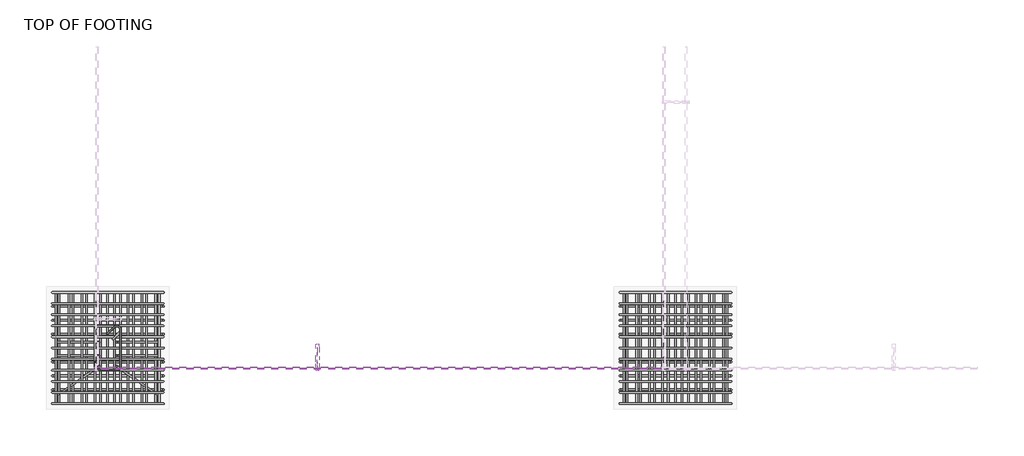
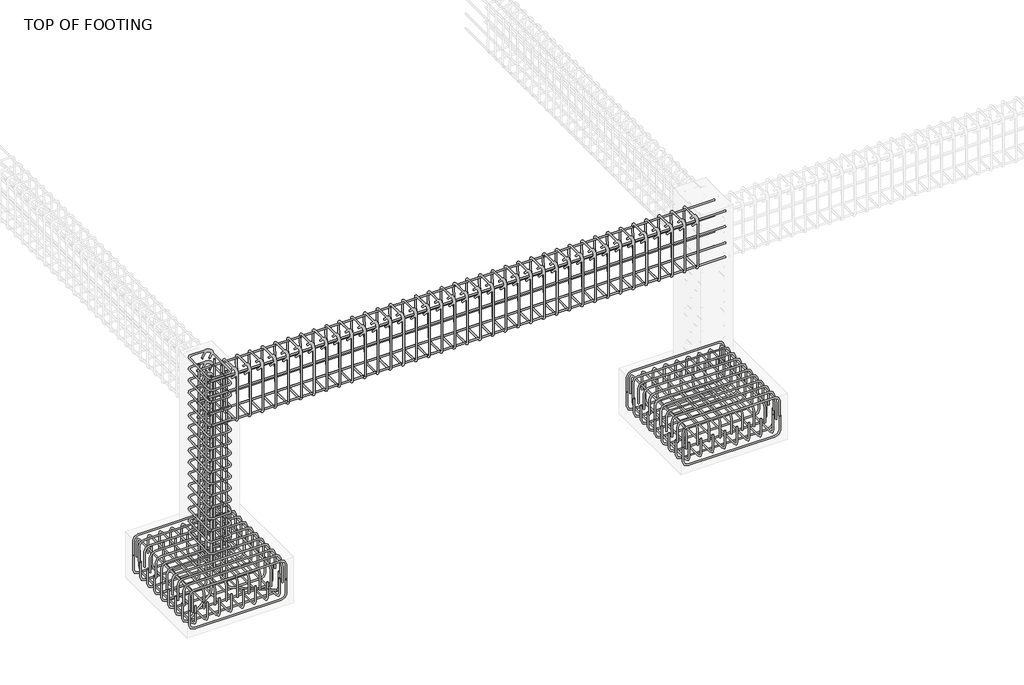
# One storey, part 2 of 13: 18 reinforcing bars.
"""IFC4 building model written with IfcOpenShell, lengths in millimetres."""

from ifc_helpers import new_model, si_unit, point, frame, origin, place, context, project, spatial, polyline, circle_curve, trimmed, segment, composite_curve, source, transform, mapped, element, save
from ifc_brep_helpers import swept_disk

model = new_model("IFC4")

# Units and contexts
model_context = context("Model", 3, world=origin())
ifc_project = project(units=[si_unit("LENGTHUNIT", "METRE", prefix="MILLI")], contexts=[model_context])

# Site, building, storey
site = spatial("IfcSite", under=ifc_project)
building = spatial("IfcBuilding", under=site)
storey = spatial("IfcBuildingStorey", under=building, Name="TOP OF FOOTING", Elevation=-1828.8)

# Reinforcing bars
placement = place(None, origin())
reinforcing_bar_shape = source(origin(), model_context, "Body", "SolidModel", [
    swept_disk(composite_curve([segment(polyline([(-6869.8542006, -3805.7842236, -2046.7304597), (-6869.8542006, -3805.7842236, -2194.0304597)]), True, "CONTINUOUS"), segment(trimmed(circle_curve(frame((-6916.2042006, -3805.7842236, -2194.0304597), z_axis=(0.0, 1.0, 0.0), x_axis=(46.350000000000364, 0.0, 0.0)), 46.35), [point((-6869.8542006, -3805.7842236, -2194.0304597))], [point((-6916.2042006, -3805.7842236, -2240.3804597))], True, "CARTESIAN"), True, "CONTINUOUS"), segment(polyline([(-6916.2042006, -3805.7842236, -2240.3804597), (-7730.8042006, -3805.7842236, -2240.3804597)]), True, "CONTINUOUS"), segment(trimmed(circle_curve(frame((-7730.8042006, -3805.7842236, -2194.0304597), z_axis=(0.0, 1.0, 0.0), x_axis=(0.0, 0.0, -46.34999999999991)), 46.35), [point((-7730.8042006, -3805.7842236, -2240.3804597))], [point((-7777.1542006, -3805.7842236, -2194.0304597))], True, "CARTESIAN"), True, "CONTINUOUS"), segment(polyline([(-7777.1542006, -3805.7842236, -2194.0304597), (-7777.1542006, -3805.7842236, -2046.7304597)]), True, "CONTINUOUS")], self_intersect=False), 6.35),
])
element("IfcReinforcingBar", 1, at=placement, inside=storey, context=model_context, shape_type="MappedRepresentation", body=[
    mapped(reinforcing_bar_shape, transform((0.0, 0.0, 0.0), x_axis=(1.0, 0.0, 0.0), y_axis=(0.0, 1.0, 0.0), z_axis=(0.0, 0.0, 1.0))),
    mapped(reinforcing_bar_shape, transform((0.0, -113.4125, 0.0), x_axis=(1.0, 0.0, 0.0), y_axis=(0.0, 1.0, 0.0), z_axis=(0.0, 0.0, 1.0))),
    mapped(reinforcing_bar_shape, transform((0.0, -226.825, 0.0), x_axis=(1.0, 0.0, 0.0), y_axis=(0.0, 1.0, 0.0), z_axis=(0.0, 0.0, 1.0))),
    mapped(reinforcing_bar_shape, transform((0.0, -340.2375, 0.0), x_axis=(1.0, 0.0, 0.0), y_axis=(0.0, 1.0, 0.0), z_axis=(0.0, 0.0, 1.0))),
    mapped(reinforcing_bar_shape, transform((0.0, -453.65, 0.0), x_axis=(1.0, 0.0, 0.0), y_axis=(0.0, 1.0, 0.0), z_axis=(0.0, 0.0, 1.0))),
    mapped(reinforcing_bar_shape, transform((0.0, -567.0625, 0.0), x_axis=(1.0, 0.0, 0.0), y_axis=(0.0, 1.0, 0.0), z_axis=(0.0, 0.0, 1.0))),
    mapped(reinforcing_bar_shape, transform((0.0, -680.475, 0.0), x_axis=(1.0, 0.0, 0.0), y_axis=(0.0, 1.0, 0.0), z_axis=(0.0, 0.0, 1.0))),
    mapped(reinforcing_bar_shape, transform((0.0, -793.8875, 0.0), x_axis=(1.0, 0.0, 0.0), y_axis=(0.0, 1.0, 0.0), z_axis=(0.0, 0.0, 1.0))),
    mapped(reinforcing_bar_shape, transform((0.0, -907.3, 0.0), x_axis=(1.0, 0.0, 0.0), y_axis=(0.0, 1.0, 0.0), z_axis=(0.0, 0.0, 1.0))),
])
reinforcing_bar_2_shape = source(origin(), model_context, "Body", "SolidModel", [
    swept_disk(composite_curve([segment(polyline([(-7777.3413042, -3805.7842236, -2054.7114114), (-7777.3413042, -3805.7842236, -1907.4114114)]), True, "CONTINUOUS"), segment(trimmed(circle_curve(frame((-7730.9913042, -3805.7842236, -1907.4114114), z_axis=(0.0, 1.0, 0.0), x_axis=(-46.350000000000364, 0.0, 0.0)), 46.35), [point((-7777.3413042, -3805.7842236, -1907.4114114))], [point((-7730.9913042, -3805.7842236, -1861.0614114))], True, "CARTESIAN"), True, "CONTINUOUS"), segment(polyline([(-7730.9913042, -3805.7842236, -1861.0614114), (-6918.3621718, -3805.7842236, -1861.0614114)]), True, "CONTINUOUS"), segment(trimmed(circle_curve(frame((-6918.3621718, -3805.7842236, -1907.4114114), z_axis=(0.0, 1.0, 0.0), x_axis=(0.0, 0.0, 46.34999999999991)), 46.35), [point((-6918.3621718, -3805.7842236, -1861.0614114))], [point((-6872.0121718, -3805.7842236, -1907.4114114))], True, "CARTESIAN"), True, "CONTINUOUS"), segment(polyline([(-6872.0121718, -3805.7842236, -1907.4114114), (-6872.0121718, -3805.7842236, -2054.7114114)]), True, "CONTINUOUS")], self_intersect=False), 6.35),
])
element("IfcReinforcingBar", 2, at=placement, inside=storey, context=model_context, shape_type="MappedRepresentation", body=[
    mapped(reinforcing_bar_2_shape, transform((0.0, 0.0, 0.0), x_axis=(1.0, 0.0, 0.0), y_axis=(0.0, 1.0, 0.0), z_axis=(0.0, 0.0, 1.0))),
    mapped(reinforcing_bar_2_shape, transform((0.0, -90.73, 0.0), x_axis=(1.0, 0.0, 0.0), y_axis=(0.0, 1.0, 0.0), z_axis=(0.0, 0.0, 1.0))),
    mapped(reinforcing_bar_2_shape, transform((0.0, -181.46, 0.0), x_axis=(1.0, 0.0, 0.0), y_axis=(0.0, 1.0, 0.0), z_axis=(0.0, 0.0, 1.0))),
    mapped(reinforcing_bar_2_shape, transform((0.0, -272.19, 0.0), x_axis=(1.0, 0.0, 0.0), y_axis=(0.0, 1.0, 0.0), z_axis=(0.0, 0.0, 1.0))),
    mapped(reinforcing_bar_2_shape, transform((0.0, -362.92, 0.0), x_axis=(1.0, 0.0, 0.0), y_axis=(0.0, 1.0, 0.0), z_axis=(0.0, 0.0, 1.0))),
    mapped(reinforcing_bar_2_shape, transform((0.0, -453.65, 0.0), x_axis=(1.0, 0.0, 0.0), y_axis=(0.0, 1.0, 0.0), z_axis=(0.0, 0.0, 1.0))),
    mapped(reinforcing_bar_2_shape, transform((0.0, -544.38, 0.0), x_axis=(1.0, 0.0, 0.0), y_axis=(0.0, 1.0, 0.0), z_axis=(0.0, 0.0, 1.0))),
    mapped(reinforcing_bar_2_shape, transform((0.0, -635.11, 0.0), x_axis=(1.0, 0.0, 0.0), y_axis=(0.0, 1.0, 0.0), z_axis=(0.0, 0.0, 1.0))),
    mapped(reinforcing_bar_2_shape, transform((0.0, -725.84, 0.0), x_axis=(1.0, 0.0, 0.0), y_axis=(0.0, 1.0, 0.0), z_axis=(0.0, 0.0, 1.0))),
    mapped(reinforcing_bar_2_shape, transform((0.0, -816.57, 0.0), x_axis=(1.0, 0.0, 0.0), y_axis=(0.0, 1.0, 0.0), z_axis=(0.0, 0.0, 1.0))),
    mapped(reinforcing_bar_2_shape, transform((0.0, -907.3, 0.0), x_axis=(1.0, 0.0, 0.0), y_axis=(0.0, 1.0, 0.0), z_axis=(0.0, 0.0, 1.0))),
])
reinforcing_bar_3_shape = source(origin(), model_context, "Body", "SolidModel", [
    swept_disk(composite_curve([segment(polyline([(-7721.4502846, -3805.7842236, -2022.6645135), (-7721.4502846, -3805.7842236, -2169.9645135)]), True, "CONTINUOUS"), segment(trimmed(circle_curve(frame((-7721.4502846, -3852.1342236, -2169.9645135), z_axis=(-1.0, 0.0, 0.0), x_axis=(0.0, 46.34999999999991, 0.0)), 46.35), [point((-7721.4502846, -3805.7842236, -2169.9645135))], [point((-7721.4502846, -3852.1342236, -2216.3145135))], True, "CARTESIAN"), True, "CONTINUOUS"), segment(polyline([(-7721.4502846, -3852.1342236, -2216.3145135), (-7721.4502846, -4666.7342236, -2216.3145135)]), True, "CONTINUOUS"), segment(trimmed(circle_curve(frame((-7721.4502846, -4666.7342236, -2169.9645135), z_axis=(-1.0, 0.0, 0.0), x_axis=(0.0, 0.0, -46.34999999999991)), 46.35), [point((-7721.4502846, -4666.7342236, -2216.3145135))], [point((-7721.4502846, -4713.0842236, -2169.9645135))], True, "CARTESIAN"), True, "CONTINUOUS"), segment(polyline([(-7721.4502846, -4713.0842236, -2169.9645135), (-7721.4502846, -4713.0842236, -2022.6645135)]), True, "CONTINUOUS")], self_intersect=False), 6.35),
])
element("IfcReinforcingBar", 3, at=placement, inside=storey, context=model_context, shape_type="MappedRepresentation", body=[
    mapped(reinforcing_bar_3_shape, transform((0.0, 0.0, 0.0), x_axis=(1.0, 0.0, 0.0), y_axis=(0.0, 1.0, 0.0), z_axis=(0.0, 0.0, 1.0))),
    mapped(reinforcing_bar_3_shape, transform((112.5551949, 0.0, 0.0), x_axis=(1.0, 0.0, 0.0), y_axis=(0.0, 1.0, 0.0), z_axis=(0.0, 0.0, 1.0))),
    mapped(reinforcing_bar_3_shape, transform((225.1103897, 0.0, 0.0), x_axis=(1.0, 0.0, 0.0), y_axis=(0.0, 1.0, 0.0), z_axis=(0.0, 0.0, 1.0))),
    mapped(reinforcing_bar_3_shape, transform((337.6655846, 0.0, 0.0), x_axis=(1.0, 0.0, 0.0), y_axis=(0.0, 1.0, 0.0), z_axis=(0.0, 0.0, 1.0))),
    mapped(reinforcing_bar_3_shape, transform((450.2207794, 0.0, 0.0), x_axis=(1.0, 0.0, 0.0), y_axis=(0.0, 1.0, 0.0), z_axis=(0.0, 0.0, 1.0))),
    mapped(reinforcing_bar_3_shape, transform((562.7759743, 0.0, 0.0), x_axis=(1.0, 0.0, 0.0), y_axis=(0.0, 1.0, 0.0), z_axis=(0.0, 0.0, 1.0))),
    mapped(reinforcing_bar_3_shape, transform((675.3311691, 0.0, 0.0), x_axis=(1.0, 0.0, 0.0), y_axis=(0.0, 1.0, 0.0), z_axis=(0.0, 0.0, 1.0))),
    mapped(reinforcing_bar_3_shape, transform((787.886364, 0.0, 0.0), x_axis=(1.0, 0.0, 0.0), y_axis=(0.0, 1.0, 0.0), z_axis=(0.0, 0.0, 1.0))),
])
reinforcing_bar_4_shape = source(origin(), model_context, "Body", "SolidModel", [
    swept_disk(composite_curve([segment(polyline([(-6905.0104502, -3805.7842236, -2073.3758937), (-6905.0104502, -3805.7842236, -1926.0758937)]), True, "CONTINUOUS"), segment(trimmed(circle_curve(frame((-6905.0104502, -3852.1342236, -1926.0758937), z_axis=(1.0, 0.0, 0.0), x_axis=(0.0, 46.34999999999991, 0.0)), 46.35), [point((-6905.0104502, -3805.7842236, -1926.0758937))], [point((-6905.0104502, -3852.1342236, -1879.7258937))], True, "CARTESIAN"), True, "CONTINUOUS"), segment(polyline([(-6905.0104502, -3852.1342236, -1879.7258937), (-6905.0104502, -4666.7342236, -1879.7258937)]), True, "CONTINUOUS"), segment(trimmed(circle_curve(frame((-6905.0104502, -4666.7342236, -1926.0758937), z_axis=(1.0, 0.0, 0.0), x_axis=(0.0, 0.0, 46.350000000000136)), 46.35), [point((-6905.0104502, -4666.7342236, -1879.7258937))], [point((-6905.0104502, -4713.0842236, -1926.0758937))], True, "CARTESIAN"), True, "CONTINUOUS"), segment(polyline([(-6905.0104502, -4713.0842236, -1926.0758937), (-6905.0104502, -4713.0842236, -2073.3758937)]), True, "CONTINUOUS")], self_intersect=False), 6.35),
])
element("IfcReinforcingBar", 4, at=placement, inside=storey, context=model_context, shape_type="MappedRepresentation", body=[
    mapped(reinforcing_bar_4_shape, transform((0.0, 0.0, 0.0), x_axis=(1.0, 0.0, 0.0), y_axis=(0.0, 1.0, 0.0), z_axis=(0.0, 0.0, 1.0))),
    mapped(reinforcing_bar_4_shape, transform((-105.0563863, 0.0, 0.0), x_axis=(1.0, 0.0, 0.0), y_axis=(0.0, 1.0, 0.0), z_axis=(0.0, 0.0, 1.0))),
    mapped(reinforcing_bar_4_shape, transform((-210.1127725, 0.0, 0.0), x_axis=(1.0, 0.0, 0.0), y_axis=(0.0, 1.0, 0.0), z_axis=(0.0, 0.0, 1.0))),
    mapped(reinforcing_bar_4_shape, transform((-315.1691588, 0.0, 0.0), x_axis=(1.0, 0.0, 0.0), y_axis=(0.0, 1.0, 0.0), z_axis=(0.0, 0.0, 1.0))),
    mapped(reinforcing_bar_4_shape, transform((-420.2255451, 0.0, 0.0), x_axis=(1.0, 0.0, 0.0), y_axis=(0.0, 1.0, 0.0), z_axis=(0.0, 0.0, 1.0))),
    mapped(reinforcing_bar_4_shape, transform((-525.2819314, 0.0, 0.0), x_axis=(1.0, 0.0, 0.0), y_axis=(0.0, 1.0, 0.0), z_axis=(0.0, 0.0, 1.0))),
    mapped(reinforcing_bar_4_shape, transform((-630.3383176, 0.0, 0.0), x_axis=(1.0, 0.0, 0.0), y_axis=(0.0, 1.0, 0.0), z_axis=(0.0, 0.0, 1.0))),
    mapped(reinforcing_bar_4_shape, transform((-735.3947039, 0.0, 0.0), x_axis=(1.0, 0.0, 0.0), y_axis=(0.0, 1.0, 0.0), z_axis=(0.0, 0.0, 1.0))),
    mapped(reinforcing_bar_4_shape, transform((-840.4510902, 0.0, 0.0), x_axis=(1.0, 0.0, 0.0), y_axis=(0.0, 1.0, 0.0), z_axis=(0.0, 0.0, 1.0))),
])
reinforcing_bar_5_shape = source(origin(), model_context, "Body", "SolidModel", [
    swept_disk(composite_curve([segment(polyline([(-2242.1090063, -3805.7842236, -2046.7304597), (-2242.1090063, -3805.7842236, -2194.0304597)]), True, "CONTINUOUS"), segment(trimmed(circle_curve(frame((-2288.4590063, -3805.7842236, -2194.0304597), z_axis=(0.0, 1.0, 0.0), x_axis=(46.34999999999991, 0.0, 0.0)), 46.35), [point((-2242.1090063, -3805.7842236, -2194.0304597))], [point((-2288.4590063, -3805.7842236, -2240.3804597))], True, "CARTESIAN"), True, "CONTINUOUS"), segment(polyline([(-2288.4590063, -3805.7842236, -2240.3804597), (-3103.0590063, -3805.7842236, -2240.3804597)]), True, "CONTINUOUS"), segment(trimmed(circle_curve(frame((-3103.0590063, -3805.7842236, -2194.0304597), z_axis=(0.0, 1.0, 0.0), x_axis=(0.0, 0.0, -46.34999999999991)), 46.35), [point((-3103.0590063, -3805.7842236, -2240.3804597))], [point((-3149.4090063, -3805.7842236, -2194.0304597))], True, "CARTESIAN"), True, "CONTINUOUS"), segment(polyline([(-3149.4090063, -3805.7842236, -2194.0304597), (-3149.4090063, -3805.7842236, -2046.7304597)]), True, "CONTINUOUS")], self_intersect=False), 6.35),
])
element("IfcReinforcingBar", 5, at=placement, inside=storey, context=model_context, shape_type="MappedRepresentation", body=[
    mapped(reinforcing_bar_5_shape, transform((0.0, 0.0, 0.0), x_axis=(1.0, 0.0, 0.0), y_axis=(0.0, 1.0, 0.0), z_axis=(0.0, 0.0, 1.0))),
    mapped(reinforcing_bar_5_shape, transform((0.0, -113.4125, 0.0), x_axis=(1.0, 0.0, 0.0), y_axis=(0.0, 1.0, 0.0), z_axis=(0.0, 0.0, 1.0))),
    mapped(reinforcing_bar_5_shape, transform((0.0, -226.825, 0.0), x_axis=(1.0, 0.0, 0.0), y_axis=(0.0, 1.0, 0.0), z_axis=(0.0, 0.0, 1.0))),
    mapped(reinforcing_bar_5_shape, transform((0.0, -340.2375, 0.0), x_axis=(1.0, 0.0, 0.0), y_axis=(0.0, 1.0, 0.0), z_axis=(0.0, 0.0, 1.0))),
    mapped(reinforcing_bar_5_shape, transform((0.0, -453.65, 0.0), x_axis=(1.0, 0.0, 0.0), y_axis=(0.0, 1.0, 0.0), z_axis=(0.0, 0.0, 1.0))),
    mapped(reinforcing_bar_5_shape, transform((0.0, -567.0625, 0.0), x_axis=(1.0, 0.0, 0.0), y_axis=(0.0, 1.0, 0.0), z_axis=(0.0, 0.0, 1.0))),
    mapped(reinforcing_bar_5_shape, transform((0.0, -680.475, 0.0), x_axis=(1.0, 0.0, 0.0), y_axis=(0.0, 1.0, 0.0), z_axis=(0.0, 0.0, 1.0))),
    mapped(reinforcing_bar_5_shape, transform((0.0, -793.8875, 0.0), x_axis=(1.0, 0.0, 0.0), y_axis=(0.0, 1.0, 0.0), z_axis=(0.0, 0.0, 1.0))),
    mapped(reinforcing_bar_5_shape, transform((0.0, -907.3, 0.0), x_axis=(1.0, 0.0, 0.0), y_axis=(0.0, 1.0, 0.0), z_axis=(0.0, 0.0, 1.0))),
])
reinforcing_bar_6_shape = source(origin(), model_context, "Body", "SolidModel", [
    swept_disk(composite_curve([segment(polyline([(-3149.5961099, -3805.7842236, -2054.7114114), (-3149.5961099, -3805.7842236, -1907.4114114)]), True, "CONTINUOUS"), segment(trimmed(circle_curve(frame((-3103.2461099, -3805.7842236, -1907.4114114), z_axis=(0.0, 1.0, 0.0), x_axis=(-46.34999999999991, 0.0, 0.0)), 46.35), [point((-3149.5961099, -3805.7842236, -1907.4114114))], [point((-3103.2461099, -3805.7842236, -1861.0614114))], True, "CARTESIAN"), True, "CONTINUOUS"), segment(polyline([(-3103.2461099, -3805.7842236, -1861.0614114), (-2290.6169775, -3805.7842236, -1861.0614114)]), True, "CONTINUOUS"), segment(trimmed(circle_curve(frame((-2290.6169775, -3805.7842236, -1907.4114114), z_axis=(0.0, 1.0, 0.0), x_axis=(0.0, 0.0, 46.34999999999991)), 46.35), [point((-2290.6169775, -3805.7842236, -1861.0614114))], [point((-2244.2669775, -3805.7842236, -1907.4114114))], True, "CARTESIAN"), True, "CONTINUOUS"), segment(polyline([(-2244.2669775, -3805.7842236, -1907.4114114), (-2244.2669775, -3805.7842236, -2054.7114114)]), True, "CONTINUOUS")], self_intersect=False), 6.35),
])
element("IfcReinforcingBar", 6, at=placement, inside=storey, context=model_context, shape_type="MappedRepresentation", body=[
    mapped(reinforcing_bar_6_shape, transform((0.0, 0.0, 0.0), x_axis=(1.0, 0.0, 0.0), y_axis=(0.0, 1.0, 0.0), z_axis=(0.0, 0.0, 1.0))),
    mapped(reinforcing_bar_6_shape, transform((0.0, -90.73, 0.0), x_axis=(1.0, 0.0, 0.0), y_axis=(0.0, 1.0, 0.0), z_axis=(0.0, 0.0, 1.0))),
    mapped(reinforcing_bar_6_shape, transform((0.0, -181.46, 0.0), x_axis=(1.0, 0.0, 0.0), y_axis=(0.0, 1.0, 0.0), z_axis=(0.0, 0.0, 1.0))),
    mapped(reinforcing_bar_6_shape, transform((0.0, -272.19, 0.0), x_axis=(1.0, 0.0, 0.0), y_axis=(0.0, 1.0, 0.0), z_axis=(0.0, 0.0, 1.0))),
    mapped(reinforcing_bar_6_shape, transform((0.0, -362.92, 0.0), x_axis=(1.0, 0.0, 0.0), y_axis=(0.0, 1.0, 0.0), z_axis=(0.0, 0.0, 1.0))),
    mapped(reinforcing_bar_6_shape, transform((0.0, -453.65, 0.0), x_axis=(1.0, 0.0, 0.0), y_axis=(0.0, 1.0, 0.0), z_axis=(0.0, 0.0, 1.0))),
    mapped(reinforcing_bar_6_shape, transform((0.0, -544.38, 0.0), x_axis=(1.0, 0.0, 0.0), y_axis=(0.0, 1.0, 0.0), z_axis=(0.0, 0.0, 1.0))),
    mapped(reinforcing_bar_6_shape, transform((0.0, -635.11, 0.0), x_axis=(1.0, 0.0, 0.0), y_axis=(0.0, 1.0, 0.0), z_axis=(0.0, 0.0, 1.0))),
    mapped(reinforcing_bar_6_shape, transform((0.0, -725.84, 0.0), x_axis=(1.0, 0.0, 0.0), y_axis=(0.0, 1.0, 0.0), z_axis=(0.0, 0.0, 1.0))),
    mapped(reinforcing_bar_6_shape, transform((0.0, -816.57, 0.0), x_axis=(1.0, 0.0, 0.0), y_axis=(0.0, 1.0, 0.0), z_axis=(0.0, 0.0, 1.0))),
    mapped(reinforcing_bar_6_shape, transform((0.0, -907.3, 0.0), x_axis=(1.0, 0.0, 0.0), y_axis=(0.0, 1.0, 0.0), z_axis=(0.0, 0.0, 1.0))),
])
reinforcing_bar_7_shape = source(origin(), model_context, "Body", "SolidModel", [
    swept_disk(composite_curve([segment(polyline([(-3093.7050902, -3805.7842236, -2022.6645135), (-3093.7050902, -3805.7842236, -2169.9645135)]), True, "CONTINUOUS"), segment(trimmed(circle_curve(frame((-3093.7050902, -3852.1342236, -2169.9645135), z_axis=(-1.0, 0.0, 0.0), x_axis=(0.0, 46.34999999999991, 0.0)), 46.35), [point((-3093.7050902, -3805.7842236, -2169.9645135))], [point((-3093.7050902, -3852.1342236, -2216.3145135))], True, "CARTESIAN"), True, "CONTINUOUS"), segment(polyline([(-3093.7050902, -3852.1342236, -2216.3145135), (-3093.7050902, -4666.7342236, -2216.3145135)]), True, "CONTINUOUS"), segment(trimmed(circle_curve(frame((-3093.7050902, -4666.7342236, -2169.9645135), z_axis=(-1.0, 0.0, 0.0), x_axis=(0.0, 0.0, -46.34999999999991)), 46.35), [point((-3093.7050902, -4666.7342236, -2216.3145135))], [point((-3093.7050902, -4713.0842236, -2169.9645135))], True, "CARTESIAN"), True, "CONTINUOUS"), segment(polyline([(-3093.7050902, -4713.0842236, -2169.9645135), (-3093.7050902, -4713.0842236, -2022.6645135)]), True, "CONTINUOUS")], self_intersect=False), 6.35),
])
element("IfcReinforcingBar", 7, at=placement, inside=storey, context=model_context, shape_type="MappedRepresentation", body=[
    mapped(reinforcing_bar_7_shape, transform((0.0, 0.0, 0.0), x_axis=(1.0, 0.0, 0.0), y_axis=(0.0, 1.0, 0.0), z_axis=(0.0, 0.0, 1.0))),
    mapped(reinforcing_bar_7_shape, transform((112.5551949, 0.0, 0.0), x_axis=(1.0, 0.0, 0.0), y_axis=(0.0, 1.0, 0.0), z_axis=(0.0, 0.0, 1.0))),
    mapped(reinforcing_bar_7_shape, transform((225.1103897, 0.0, 0.0), x_axis=(1.0, 0.0, 0.0), y_axis=(0.0, 1.0, 0.0), z_axis=(0.0, 0.0, 1.0))),
    mapped(reinforcing_bar_7_shape, transform((337.6655846, 0.0, 0.0), x_axis=(1.0, 0.0, 0.0), y_axis=(0.0, 1.0, 0.0), z_axis=(0.0, 0.0, 1.0))),
    mapped(reinforcing_bar_7_shape, transform((450.2207794, 0.0, 0.0), x_axis=(1.0, 0.0, 0.0), y_axis=(0.0, 1.0, 0.0), z_axis=(0.0, 0.0, 1.0))),
    mapped(reinforcing_bar_7_shape, transform((562.7759743, 0.0, 0.0), x_axis=(1.0, 0.0, 0.0), y_axis=(0.0, 1.0, 0.0), z_axis=(0.0, 0.0, 1.0))),
    mapped(reinforcing_bar_7_shape, transform((675.3311691, 0.0, 0.0), x_axis=(1.0, 0.0, 0.0), y_axis=(0.0, 1.0, 0.0), z_axis=(0.0, 0.0, 1.0))),
    mapped(reinforcing_bar_7_shape, transform((787.886364, 0.0, 0.0), x_axis=(1.0, 0.0, 0.0), y_axis=(0.0, 1.0, 0.0), z_axis=(0.0, 0.0, 1.0))),
])
reinforcing_bar_8_shape = source(origin(), model_context, "Body", "SolidModel", [
    swept_disk(composite_curve([segment(polyline([(-2277.2652559, -3805.7842236, -2073.3758937), (-2277.2652559, -3805.7842236, -1926.0758937)]), True, "CONTINUOUS"), segment(trimmed(circle_curve(frame((-2277.2652559, -3852.1342236, -1926.0758937), z_axis=(1.0, 0.0, 0.0), x_axis=(0.0, 46.34999999999991, 0.0)), 46.35), [point((-2277.2652559, -3805.7842236, -1926.0758937))], [point((-2277.2652559, -3852.1342236, -1879.7258937))], True, "CARTESIAN"), True, "CONTINUOUS"), segment(polyline([(-2277.2652559, -3852.1342236, -1879.7258937), (-2277.2652559, -4666.7342236, -1879.7258937)]), True, "CONTINUOUS"), segment(trimmed(circle_curve(frame((-2277.2652559, -4666.7342236, -1926.0758937), z_axis=(1.0, 0.0, 0.0), x_axis=(0.0, 0.0, 46.350000000000136)), 46.35), [point((-2277.2652559, -4666.7342236, -1879.7258937))], [point((-2277.2652559, -4713.0842236, -1926.0758937))], True, "CARTESIAN"), True, "CONTINUOUS"), segment(polyline([(-2277.2652559, -4713.0842236, -1926.0758937), (-2277.2652559, -4713.0842236, -2073.3758937)]), True, "CONTINUOUS")], self_intersect=False), 6.35),
])
element("IfcReinforcingBar", 8, at=placement, inside=storey, context=model_context, shape_type="MappedRepresentation", body=[
    mapped(reinforcing_bar_8_shape, transform((0.0, 0.0, 0.0), x_axis=(1.0, 0.0, 0.0), y_axis=(0.0, 1.0, 0.0), z_axis=(0.0, 0.0, 1.0))),
    mapped(reinforcing_bar_8_shape, transform((-105.0563863, 0.0, 0.0), x_axis=(1.0, 0.0, 0.0), y_axis=(0.0, 1.0, 0.0), z_axis=(0.0, 0.0, 1.0))),
    mapped(reinforcing_bar_8_shape, transform((-210.1127725, 0.0, 0.0), x_axis=(1.0, 0.0, 0.0), y_axis=(0.0, 1.0, 0.0), z_axis=(0.0, 0.0, 1.0))),
    mapped(reinforcing_bar_8_shape, transform((-315.1691588, 0.0, 0.0), x_axis=(1.0, 0.0, 0.0), y_axis=(0.0, 1.0, 0.0), z_axis=(0.0, 0.0, 1.0))),
    mapped(reinforcing_bar_8_shape, transform((-420.2255451, 0.0, 0.0), x_axis=(1.0, 0.0, 0.0), y_axis=(0.0, 1.0, 0.0), z_axis=(0.0, 0.0, 1.0))),
    mapped(reinforcing_bar_8_shape, transform((-525.2819314, 0.0, 0.0), x_axis=(1.0, 0.0, 0.0), y_axis=(0.0, 1.0, 0.0), z_axis=(0.0, 0.0, 1.0))),
    mapped(reinforcing_bar_8_shape, transform((-630.3383176, 0.0, 0.0), x_axis=(1.0, 0.0, 0.0), y_axis=(0.0, 1.0, 0.0), z_axis=(0.0, 0.0, 1.0))),
    mapped(reinforcing_bar_8_shape, transform((-735.3947039, 0.0, 0.0), x_axis=(1.0, 0.0, 0.0), y_axis=(0.0, 1.0, 0.0), z_axis=(0.0, 0.0, 1.0))),
    mapped(reinforcing_bar_8_shape, transform((-840.4510902, 0.0, 0.0), x_axis=(1.0, 0.0, 0.0), y_axis=(0.0, 1.0, 0.0), z_axis=(0.0, 0.0, 1.0))),
])
reinforcing_bar_9_shape = source(origin(), model_context, "Body", "SolidModel", [
    swept_disk(composite_curve([segment(polyline([(-7329.1155612, -4145.7099889, -46.35), (-7273.3719982, -4089.966426, -46.35)]), True, "CONTINUOUS"), segment(trimmed(circle_curve(frame((-7251.2042006, -4112.1342236, -46.35), z_axis=(0.0, 0.0, -1.0), x_axis=(-22.167797600000085, 22.167797600000085, 0.0)), 31.35), [point((-7273.3719982, -4089.966426, -46.35))], [point((-7219.8542006, -4112.1342236, -46.35))], True, "CARTESIAN"), True, "CONTINUOUS"), segment(polyline([(-7219.8542006, -4112.1342236, -46.35), (-7219.8542006, -4406.7342236, -46.35)]), True, "CONTINUOUS"), segment(trimmed(circle_curve(frame((-7251.2042006, -4406.7342236, -46.35), z_axis=(0.0, 0.0, -1.0), x_axis=(31.350000000000364, 0.0, 0.0)), 31.35), [point((-7219.8542006, -4406.7342236, -46.35))], [point((-7251.2042006, -4438.0842236, -46.35))], True, "CARTESIAN"), True, "CONTINUOUS"), segment(polyline([(-7251.2042006, -4438.0842236, -46.35), (-7395.8042006, -4438.0842236, -46.35)]), True, "CONTINUOUS"), segment(trimmed(circle_curve(frame((-7395.8042006, -4406.7540087, -45.2363875), z_axis=(0.0, 0.035521928334481916, -0.9993688971583016), x_axis=(0.0, -31.3302149000001, -1.1136125000000021)), 31.35), [point((-7395.8042006, -4438.0842236, -46.35))], [point((-7427.1542006, -4406.7540087, -45.2363875))], True, "CARTESIAN"), True, "CONTINUOUS"), segment(polyline([(-7427.1542006, -4406.7540087, -45.2363875), (-7427.1542006, -4112.1144385, -34.7636125)]), True, "CONTINUOUS"), segment(trimmed(circle_curve(frame((-7395.8042006, -4112.1144385, -34.7636125), z_axis=(0.0, 0.035521928334481916, -0.9993688971583016), x_axis=(-31.350000000000364, 0.0, 0.0)), 31.35), [point((-7427.1542006, -4112.1144385, -34.7636125))], [point((-7395.8042006, -4080.7842236, -33.65))], True, "CARTESIAN"), True, "CONTINUOUS"), segment(polyline([(-7395.8042006, -4080.7842236, -33.65), (-7251.2042006, -4080.7842236, -33.65)]), True, "CONTINUOUS"), segment(trimmed(circle_curve(frame((-7251.2042006, -4112.1342236, -33.65), z_axis=(0.0, 0.0, -1.0), x_axis=(0.0, 31.34999999999991, 0.0)), 31.35), [point((-7251.2042006, -4080.7842236, -33.65))], [point((-7229.036403, -4134.3020212, -33.65))], True, "CARTESIAN"), True, "CONTINUOUS"), segment(polyline([(-7229.036403, -4134.3020212, -33.65), (-7284.779966, -4190.0455841, -33.65)]), True, "CONTINUOUS")], self_intersect=False), 6.35),
])
element("IfcReinforcingBar", 9, at=placement, inside=storey, context=model_context, shape_type="MappedRepresentation", body=[
    mapped(reinforcing_bar_9_shape, transform((0.0, 0.0, 0.0), x_axis=(1.0, 0.0, 0.0), y_axis=(0.0, 1.0, 0.0), z_axis=(0.0, 0.0, 1.0))),
    mapped(reinforcing_bar_9_shape, transform((0.0, 0.0, -115.74), x_axis=(1.0, 0.0, 0.0), y_axis=(0.0, 1.0, 0.0), z_axis=(0.0, 0.0, 1.0))),
    mapped(reinforcing_bar_9_shape, transform((0.0, 0.0, -231.48), x_axis=(1.0, 0.0, 0.0), y_axis=(0.0, 1.0, 0.0), z_axis=(0.0, 0.0, 1.0))),
    mapped(reinforcing_bar_9_shape, transform((0.0, 0.0, -347.22), x_axis=(1.0, 0.0, 0.0), y_axis=(0.0, 1.0, 0.0), z_axis=(0.0, 0.0, 1.0))),
    mapped(reinforcing_bar_9_shape, transform((0.0, 0.0, -462.96), x_axis=(1.0, 0.0, 0.0), y_axis=(0.0, 1.0, 0.0), z_axis=(0.0, 0.0, 1.0))),
    mapped(reinforcing_bar_9_shape, transform((0.0, 0.0, -578.7), x_axis=(1.0, 0.0, 0.0), y_axis=(0.0, 1.0, 0.0), z_axis=(0.0, 0.0, 1.0))),
    mapped(reinforcing_bar_9_shape, transform((0.0, 0.0, -694.44), x_axis=(1.0, 0.0, 0.0), y_axis=(0.0, 1.0, 0.0), z_axis=(0.0, 0.0, 1.0))),
    mapped(reinforcing_bar_9_shape, transform((0.0, 0.0, -810.18), x_axis=(1.0, 0.0, 0.0), y_axis=(0.0, 1.0, 0.0), z_axis=(0.0, 0.0, 1.0))),
    mapped(reinforcing_bar_9_shape, transform((0.0, 0.0, -925.92), x_axis=(1.0, 0.0, 0.0), y_axis=(0.0, 1.0, 0.0), z_axis=(0.0, 0.0, 1.0))),
    mapped(reinforcing_bar_9_shape, transform((0.0, 0.0, -1041.66), x_axis=(1.0, 0.0, 0.0), y_axis=(0.0, 1.0, 0.0), z_axis=(0.0, 0.0, 1.0))),
    mapped(reinforcing_bar_9_shape, transform((0.0, 0.0, -1157.4), x_axis=(1.0, 0.0, 0.0), y_axis=(0.0, 1.0, 0.0), z_axis=(0.0, 0.0, 1.0))),
    mapped(reinforcing_bar_9_shape, transform((0.0, 0.0, -1273.14), x_axis=(1.0, 0.0, 0.0), y_axis=(0.0, 1.0, 0.0), z_axis=(0.0, 0.0, 1.0))),
    mapped(reinforcing_bar_9_shape, transform((0.0, 0.0, -1388.88), x_axis=(1.0, 0.0, 0.0), y_axis=(0.0, 1.0, 0.0), z_axis=(0.0, 0.0, 1.0))),
    mapped(reinforcing_bar_9_shape, transform((0.0, 0.0, -1504.62), x_axis=(1.0, 0.0, 0.0), y_axis=(0.0, 1.0, 0.0), z_axis=(0.0, 0.0, 1.0))),
    mapped(reinforcing_bar_9_shape, transform((0.0, 0.0, -1620.36), x_axis=(1.0, 0.0, 0.0), y_axis=(0.0, 1.0, 0.0), z_axis=(0.0, 0.0, 1.0))),
    mapped(reinforcing_bar_9_shape, transform((0.0, 0.0, -1736.1), x_axis=(1.0, 0.0, 0.0), y_axis=(0.0, 1.0, 0.0), z_axis=(0.0, 0.0, 1.0))),
])
element("IfcReinforcingBar", 10, at=placement, inside=storey, context=model_context, shape_type="SolidModel", body=[
    swept_disk(composite_curve([segment(polyline([(-7251.2042006, -4408.0347869, -40.0), (-7251.2042006, -4408.0347869, -2142.45)]), True, "CONTINUOUS"), segment(trimmed(circle_curve(frame((-7213.2365034, -4434.6200547, -2142.45), z_axis=(-0.5735764363510132, -0.8191520442890149, 0.0), x_axis=(-37.96769719999975, 26.58526780000011, 0.0)), 46.35), [point((-7251.2042006, -4408.0347869, -2142.45))], [point((-7213.2365034, -4434.6200547, -2188.8))], True, "CARTESIAN"), True, "CONTINUOUS"), segment(polyline([(-7213.2365034, -4434.6200547, -2188.8), (-6917.2359122, -4641.8819, -2188.8)]), True, "CONTINUOUS")], self_intersect=False), 6.35),
])
element("IfcReinforcingBar", 11, at=placement, inside=storey, context=model_context, shape_type="SolidModel", body=[
    swept_disk(composite_curve([segment(polyline([(-7395.8042006, -4408.0347869, -40.0), (-7395.8042006, -4408.0347869, -2142.45)]), True, "CONTINUOUS"), segment(trimmed(circle_curve(frame((-7433.7718979, -4434.6200547, -2142.45), z_axis=(-0.5735764363510413, 0.8191520442889952, 0.0), x_axis=(37.96769730000051, 26.58526780000011, 0.0)), 46.35), [point((-7395.8042006, -4408.0347869, -2142.45))], [point((-7433.7718979, -4434.6200547, -2188.8))], True, "CARTESIAN"), True, "CONTINUOUS"), segment(polyline([(-7433.7718979, -4434.6200547, -2188.8), (-7729.7724891, -4641.8819, -2188.8)]), True, "CONTINUOUS")], self_intersect=False), 6.35),
])
reinforcing_bar_10_shape = source(origin(), model_context, "Body", "SolidModel", [
    swept_disk(composite_curve([segment(polyline([(-7395.8042006, -4212.4451378, -40.0), (-7395.8042006, -4212.4451378, -2135.3077585)]), True, "CONTINUOUS"), segment(trimmed(circle_curve(frame((-7442.1542006, -4212.4451378, -2135.3077585), z_axis=(0.0, 1.0, 0.0), x_axis=(46.350000000000364, 0.0, 0.0)), 46.35), [point((-7395.8042006, -4212.4451378, -2135.3077585))], [point((-7442.1542006, -4212.4451378, -2181.6577585))], True, "CARTESIAN"), True, "CONTINUOUS"), segment(polyline([(-7442.1542006, -4212.4451378, -2181.6577585), (-7738.4759323, -4212.4451378, -2181.6577585)]), True, "CONTINUOUS")], self_intersect=False), 6.35),
])
element("IfcReinforcingBar", 12, at=placement, inside=storey, context=model_context, shape_type="MappedRepresentation", body=[
    mapped(reinforcing_bar_10_shape, transform((0.0, 0.0, 0.0), x_axis=(1.0, 0.0, 0.0), y_axis=(0.0, 1.0, 0.0), z_axis=(0.0, 0.0, 1.0))),
    mapped(reinforcing_bar_10_shape, transform((0.0, -110.4020916, 0.0), x_axis=(1.0, 0.0, 0.0), y_axis=(0.0, 1.0, 0.0), z_axis=(0.0, 0.0, 1.0))),
])
reinforcing_bar_11_shape = source(origin(), model_context, "Body", "SolidModel", [
    swept_disk(composite_curve([segment(polyline([(-7251.2042006, -4212.4451378, -40.0), (-7251.2042006, -4212.4451378, -2135.3077585)]), True, "CONTINUOUS"), segment(trimmed(circle_curve(frame((-7204.8542006, -4212.4451378, -2135.3077585), z_axis=(0.0, -1.0, 0.0), x_axis=(-46.350000000000364, 0.0, 0.0)), 46.35), [point((-7251.2042006, -4212.4451378, -2135.3077585))], [point((-7204.8542006, -4212.4451378, -2181.6577585))], True, "CARTESIAN"), True, "CONTINUOUS"), segment(polyline([(-7204.8542006, -4212.4451378, -2181.6577585), (-6908.532469, -4212.4451378, -2181.6577585)]), True, "CONTINUOUS")], self_intersect=False), 6.35),
])
element("IfcReinforcingBar", 13, at=placement, inside=storey, context=model_context, shape_type="MappedRepresentation", body=[
    mapped(reinforcing_bar_11_shape, transform((0.0, 0.0, 0.0), x_axis=(1.0, 0.0, 0.0), y_axis=(0.0, 1.0, 0.0), z_axis=(0.0, 0.0, 1.0))),
    mapped(reinforcing_bar_11_shape, transform((0.0, -110.4020916, 0.0), x_axis=(1.0, 0.0, 0.0), y_axis=(0.0, 1.0, 0.0), z_axis=(0.0, 0.0, 1.0))),
])
reinforcing_bar_12_shape = source(origin(), model_context, "Body", "SolidModel", [
    swept_disk(composite_curve([segment(polyline([(-7167.1542006, -4328.822863, -111.2757654), (-7167.1542006, -4384.566426, -55.5322024)]), True, "CONTINUOUS"), segment(trimmed(circle_curve(frame((-7167.1542006, -4406.7342236, -77.7), z_axis=(1.0, 0.0, 0.0), x_axis=(0.0, 22.167797600000085, 22.1677976)), 31.35), [point((-7167.1542006, -4384.566426, -55.5322024))], [point((-7167.1542006, -4438.0842236, -77.7))], True, "CARTESIAN"), True, "CONTINUOUS"), segment(polyline([(-7167.1542006, -4438.0842236, -77.7), (-7167.1542006, -4438.0842236, -522.3)]), True, "CONTINUOUS"), segment(trimmed(circle_curve(frame((-7167.1542006, -4406.7342236, -522.3), z_axis=(1.0, 0.0, 0.0), x_axis=(0.0, -31.349999999999454, 0.0)), 31.35), [point((-7167.1542006, -4438.0842236, -522.3))], [point((-7167.1542006, -4406.7342236, -553.65))], True, "CARTESIAN"), True, "CONTINUOUS"), segment(polyline([(-7167.1542006, -4406.7342236, -553.65), (-7167.1542006, -4262.1342236, -553.65)]), True, "CONTINUOUS"), segment(trimmed(circle_curve(frame((-7167.9387863, -4262.1342236, -522.3098193), z_axis=(0.9996867842138424, 0.0, 0.02502665515378633), x_axis=(0.784585700000207, 0.0, -31.34018070000002)), 31.35), [point((-7167.1542006, -4262.1342236, -553.65))], [point((-7167.9387863, -4230.7842236, -522.3098193))], True, "CARTESIAN"), True, "CONTINUOUS"), segment(polyline([(-7167.9387863, -4230.7842236, -522.3098193), (-7179.069615, -4230.7842236, -77.6901807)]), True, "CONTINUOUS"), segment(trimmed(circle_curve(frame((-7179.069615, -4262.1342236, -77.6901807), z_axis=(0.9996867842138424, 0.0, 0.02502665515378633), x_axis=(0.0, 31.350000000000364, 0.0)), 31.35), [point((-7179.069615, -4230.7842236, -77.6901807))], [point((-7179.8542006, -4262.1342236, -46.35))], True, "CARTESIAN"), True, "CONTINUOUS"), segment(polyline([(-7179.8542006, -4262.1342236, -46.35), (-7179.8542006, -4406.7342236, -46.35)]), True, "CONTINUOUS"), segment(trimmed(circle_curve(frame((-7179.8542006, -4406.7342236, -77.7), z_axis=(1.0, 0.0, 0.0), x_axis=(0.0, 0.0, 31.35)), 31.35), [point((-7179.8542006, -4406.7342236, -46.35))], [point((-7179.8542006, -4428.9020212, -99.8677976))], True, "CARTESIAN"), True, "CONTINUOUS"), segment(polyline([(-7179.8542006, -4428.9020212, -99.8677976), (-7179.8542006, -4373.1584582, -155.6113605)]), True, "CONTINUOUS")], self_intersect=False), 6.35),
])
element("IfcReinforcingBar", 14, at=placement, inside=storey, context=model_context, shape_type="MappedRepresentation", body=[
    mapped(reinforcing_bar_12_shape, transform((0.0, 0.0, 0.0), x_axis=(1.0, 0.0, 0.0), y_axis=(0.0, 1.0, 0.0), z_axis=(0.0, 0.0, 1.0))),
    mapped(reinforcing_bar_12_shape, transform((119.8623665, 0.0, 0.0), x_axis=(1.0, 0.0, 0.0), y_axis=(0.0, 1.0, 0.0), z_axis=(0.0, 0.0, 1.0))),
    mapped(reinforcing_bar_12_shape, transform((239.724733, 0.0, 0.0), x_axis=(1.0, 0.0, 0.0), y_axis=(0.0, 1.0, 0.0), z_axis=(0.0, 0.0, 1.0))),
    mapped(reinforcing_bar_12_shape, transform((359.5870995, 0.0, 0.0), x_axis=(1.0, 0.0, 0.0), y_axis=(0.0, 1.0, 0.0), z_axis=(0.0, 0.0, 1.0))),
    mapped(reinforcing_bar_12_shape, transform((479.449466, 0.0, 0.0), x_axis=(1.0, 0.0, 0.0), y_axis=(0.0, 1.0, 0.0), z_axis=(0.0, 0.0, 1.0))),
    mapped(reinforcing_bar_12_shape, transform((599.3118325, 0.0, 0.0), x_axis=(1.0, 0.0, 0.0), y_axis=(0.0, 1.0, 0.0), z_axis=(0.0, 0.0, 1.0))),
    mapped(reinforcing_bar_12_shape, transform((719.1741991, 0.0, 0.0), x_axis=(1.0, 0.0, 0.0), y_axis=(0.0, 1.0, 0.0), z_axis=(0.0, 0.0, 1.0))),
    mapped(reinforcing_bar_12_shape, transform((839.0365656, 0.0, 0.0), x_axis=(1.0, 0.0, 0.0), y_axis=(0.0, 1.0, 0.0), z_axis=(0.0, 0.0, 1.0))),
    mapped(reinforcing_bar_12_shape, transform((958.8989321, 0.0, 0.0), x_axis=(1.0, 0.0, 0.0), y_axis=(0.0, 1.0, 0.0), z_axis=(0.0, 0.0, 1.0))),
    mapped(reinforcing_bar_12_shape, transform((1078.7612986, 0.0, 0.0), x_axis=(1.0, 0.0, 0.0), y_axis=(0.0, 1.0, 0.0), z_axis=(0.0, 0.0, 1.0))),
    mapped(reinforcing_bar_12_shape, transform((1198.6236651, 0.0, 0.0), x_axis=(1.0, 0.0, 0.0), y_axis=(0.0, 1.0, 0.0), z_axis=(0.0, 0.0, 1.0))),
    mapped(reinforcing_bar_12_shape, transform((1318.4860316, 0.0, 0.0), x_axis=(1.0, 0.0, 0.0), y_axis=(0.0, 1.0, 0.0), z_axis=(0.0, 0.0, 1.0))),
    mapped(reinforcing_bar_12_shape, transform((1438.3483981, 0.0, 0.0), x_axis=(1.0, 0.0, 0.0), y_axis=(0.0, 1.0, 0.0), z_axis=(0.0, 0.0, 1.0))),
    mapped(reinforcing_bar_12_shape, transform((1558.2107646, 0.0, 0.0), x_axis=(1.0, 0.0, 0.0), y_axis=(0.0, 1.0, 0.0), z_axis=(0.0, 0.0, 1.0))),
    mapped(reinforcing_bar_12_shape, transform((1678.0731311, 0.0, 0.0), x_axis=(1.0, 0.0, 0.0), y_axis=(0.0, 1.0, 0.0), z_axis=(0.0, 0.0, 1.0))),
    mapped(reinforcing_bar_12_shape, transform((1797.9354976, 0.0, 0.0), x_axis=(1.0, 0.0, 0.0), y_axis=(0.0, 1.0, 0.0), z_axis=(0.0, 0.0, 1.0))),
    mapped(reinforcing_bar_12_shape, transform((1917.7978642, 0.0, 0.0), x_axis=(1.0, 0.0, 0.0), y_axis=(0.0, 1.0, 0.0), z_axis=(0.0, 0.0, 1.0))),
    mapped(reinforcing_bar_12_shape, transform((2037.6602307, 0.0, 0.0), x_axis=(1.0, 0.0, 0.0), y_axis=(0.0, 1.0, 0.0), z_axis=(0.0, 0.0, 1.0))),
    mapped(reinforcing_bar_12_shape, transform((2157.5225972, 0.0, 0.0), x_axis=(1.0, 0.0, 0.0), y_axis=(0.0, 1.0, 0.0), z_axis=(0.0, 0.0, 1.0))),
    mapped(reinforcing_bar_12_shape, transform((2277.3849637, 0.0, 0.0), x_axis=(1.0, 0.0, 0.0), y_axis=(0.0, 1.0, 0.0), z_axis=(0.0, 0.0, 1.0))),
    mapped(reinforcing_bar_12_shape, transform((2397.2473302, 0.0, 0.0), x_axis=(1.0, 0.0, 0.0), y_axis=(0.0, 1.0, 0.0), z_axis=(0.0, 0.0, 1.0))),
    mapped(reinforcing_bar_12_shape, transform((2517.1096967, 0.0, 0.0), x_axis=(1.0, 0.0, 0.0), y_axis=(0.0, 1.0, 0.0), z_axis=(0.0, 0.0, 1.0))),
    mapped(reinforcing_bar_12_shape, transform((2636.9720632, 0.0, 0.0), x_axis=(1.0, 0.0, 0.0), y_axis=(0.0, 1.0, 0.0), z_axis=(0.0, 0.0, 1.0))),
    mapped(reinforcing_bar_12_shape, transform((2756.8344297, 0.0, 0.0), x_axis=(1.0, 0.0, 0.0), y_axis=(0.0, 1.0, 0.0), z_axis=(0.0, 0.0, 1.0))),
    mapped(reinforcing_bar_12_shape, transform((2876.6967962, 0.0, 0.0), x_axis=(1.0, 0.0, 0.0), y_axis=(0.0, 1.0, 0.0), z_axis=(0.0, 0.0, 1.0))),
    mapped(reinforcing_bar_12_shape, transform((2996.5591627, 0.0, 0.0), x_axis=(1.0, 0.0, 0.0), y_axis=(0.0, 1.0, 0.0), z_axis=(0.0, 0.0, 1.0))),
    mapped(reinforcing_bar_12_shape, transform((3116.4215293, 0.0, 0.0), x_axis=(1.0, 0.0, 0.0), y_axis=(0.0, 1.0, 0.0), z_axis=(0.0, 0.0, 1.0))),
    mapped(reinforcing_bar_12_shape, transform((3236.2838958, 0.0, 0.0), x_axis=(1.0, 0.0, 0.0), y_axis=(0.0, 1.0, 0.0), z_axis=(0.0, 0.0, 1.0))),
    mapped(reinforcing_bar_12_shape, transform((3356.1462623, 0.0, 0.0), x_axis=(1.0, 0.0, 0.0), y_axis=(0.0, 1.0, 0.0), z_axis=(0.0, 0.0, 1.0))),
    mapped(reinforcing_bar_12_shape, transform((3476.0086288, 0.0, 0.0), x_axis=(1.0, 0.0, 0.0), y_axis=(0.0, 1.0, 0.0), z_axis=(0.0, 0.0, 1.0))),
    mapped(reinforcing_bar_12_shape, transform((3595.8709953, 0.0, 0.0), x_axis=(1.0, 0.0, 0.0), y_axis=(0.0, 1.0, 0.0), z_axis=(0.0, 0.0, 1.0))),
    mapped(reinforcing_bar_12_shape, transform((3715.7333618, 0.0, 0.0), x_axis=(1.0, 0.0, 0.0), y_axis=(0.0, 1.0, 0.0), z_axis=(0.0, 0.0, 1.0))),
    mapped(reinforcing_bar_12_shape, transform((3835.5957283, 0.0, 0.0), x_axis=(1.0, 0.0, 0.0), y_axis=(0.0, 1.0, 0.0), z_axis=(0.0, 0.0, 1.0))),
    mapped(reinforcing_bar_12_shape, transform((3955.4580948, 0.0, 0.0), x_axis=(1.0, 0.0, 0.0), y_axis=(0.0, 1.0, 0.0), z_axis=(0.0, 0.0, 1.0))),
    mapped(reinforcing_bar_12_shape, transform((4075.3204613, 0.0, 0.0), x_axis=(1.0, 0.0, 0.0), y_axis=(0.0, 1.0, 0.0), z_axis=(0.0, 0.0, 1.0))),
    mapped(reinforcing_bar_12_shape, transform((4195.1828278, 0.0, 0.0), x_axis=(1.0, 0.0, 0.0), y_axis=(0.0, 1.0, 0.0), z_axis=(0.0, 0.0, 1.0))),
    mapped(reinforcing_bar_12_shape, transform((4315.0451944, 0.0, 0.0), x_axis=(1.0, 0.0, 0.0), y_axis=(0.0, 1.0, 0.0), z_axis=(0.0, 0.0, 1.0))),
])
reinforcing_bar_13_shape = source(origin(), model_context, "Body", "SolidModel", [
    swept_disk(composite_curve([segment(polyline([(-7433.5042006, -4243.4842236, -77.7), (-2585.7590063, -4243.4842236, -77.7)]), True, "CONTINUOUS")], self_intersect=False), 6.35),
])
element("IfcReinforcingBar", 15, at=placement, inside=storey, context=model_context, shape_type="MappedRepresentation", body=[
    mapped(reinforcing_bar_13_shape, transform((0.0, 0.0, 0.0), x_axis=(1.0, 0.0, 0.0), y_axis=(0.0, 1.0, 0.0), z_axis=(0.0, 0.0, 1.0))),
    mapped(reinforcing_bar_13_shape, transform((0.0, -181.9, 0.0), x_axis=(1.0, 0.0, 0.0), y_axis=(0.0, 1.0, 0.0), z_axis=(0.0, 0.0, 1.0))),
])
reinforcing_bar_14_shape = source(origin(), model_context, "Body", "SolidModel", [
    swept_disk(composite_curve([segment(polyline([(-7433.5042006, -4248.9466821, -535.4875415), (-2585.7590063, -4248.9466821, -535.4875415)]), True, "CONTINUOUS")], self_intersect=False), 6.35),
])
element("IfcReinforcingBar", 16, at=placement, inside=storey, context=model_context, shape_type="MappedRepresentation", body=[
    mapped(reinforcing_bar_14_shape, transform((0.0, 0.0, 0.0), x_axis=(1.0, 0.0, 0.0), y_axis=(0.0, 1.0, 0.0), z_axis=(0.0, 0.0, 1.0))),
    mapped(reinforcing_bar_14_shape, transform((0.0, -170.9750829, 0.0), x_axis=(1.0, 0.0, 0.0), y_axis=(0.0, 1.0, 0.0), z_axis=(0.0, 0.0, 1.0))),
])
reinforcing_bar_15_shape = source(origin(), model_context, "Body", "SolidModel", [
    swept_disk(composite_curve([segment(polyline([(-7433.5042006, -4243.4842236, -392.3), (-2585.7590063, -4243.4842236, -392.3)]), True, "CONTINUOUS")], self_intersect=False), 6.35),
])
element("IfcReinforcingBar", 17, at=placement, inside=storey, context=model_context, shape_type="MappedRepresentation", body=[
    mapped(reinforcing_bar_15_shape, transform((0.0, 0.0, 0.0), x_axis=(1.0, 0.0, 0.0), y_axis=(0.0, 1.0, 0.0), z_axis=(0.0, 0.0, 1.0))),
    mapped(reinforcing_bar_15_shape, transform((0.0, -182.177358, 0.0), x_axis=(1.0, 0.0, 0.0), y_axis=(0.0, 1.0, 0.0), z_axis=(0.0, 0.0, 1.0))),
])
reinforcing_bar_16_shape = source(origin(), model_context, "Body", "SolidModel", [
    swept_disk(composite_curve([segment(polyline([(-7433.5042006, -4243.4842236, -232.3), (-2585.7590063, -4243.4842236, -232.3)]), True, "CONTINUOUS")], self_intersect=False), 6.35),
])
element("IfcReinforcingBar", 18, at=placement, inside=storey, context=model_context, shape_type="MappedRepresentation", body=[
    mapped(reinforcing_bar_16_shape, transform((0.0, 0.0, 0.0), x_axis=(1.0, 0.0, 0.0), y_axis=(0.0, 1.0, 0.0), z_axis=(0.0, 0.0, 1.0))),
    mapped(reinforcing_bar_16_shape, transform((0.0, -182.177358, 0.0), x_axis=(1.0, 0.0, 0.0), y_axis=(0.0, 1.0, 0.0), z_axis=(0.0, 0.0, 1.0))),
])

save(model, "model.ifc")

# Revit data of these elements
# Elements 1, 2, 3, 4, 5, 6, 7, 8, 9, 10, 11, 12, 13, 14, 15, 16, 17, 18 (IfcReinforcingBar)
#   Phase Created = New Construction
